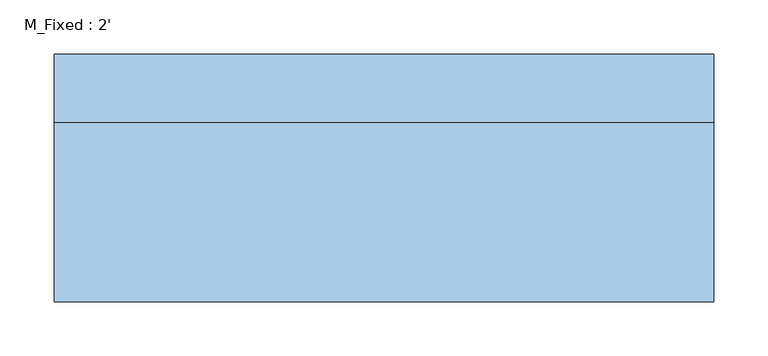
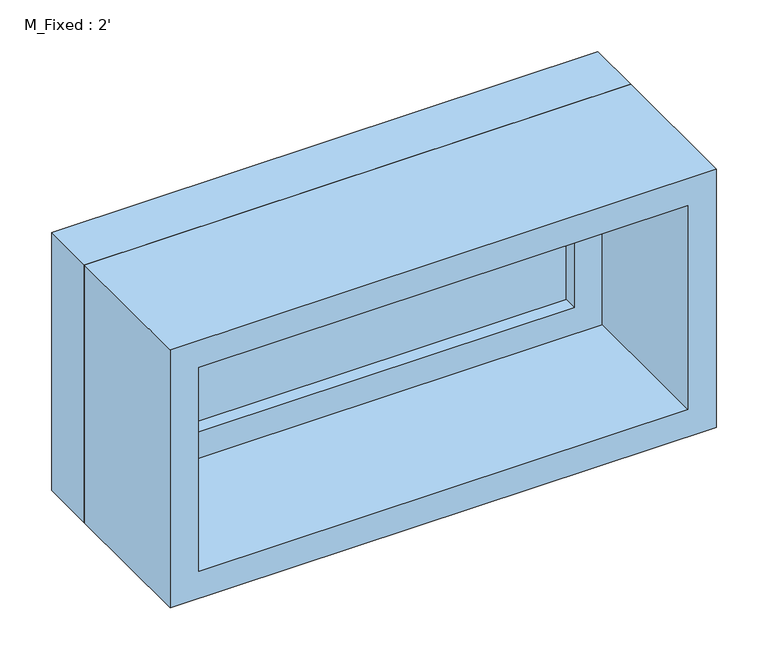
"""IFC4 building model written with IfcOpenShell, lengths in millimetres: window geometry, M_Fixed : 2'."""

from ifc_helpers import new_model, si_unit, frame, origin, place, context, project, spatial, polyline, outline, extrude, source, transform, mapped, element, save


def m_fixed_2_dd9f9b20(model_context):
    return source(origin(), model_context, "Body", "SweptSolid", [
        extrude(outline(polyline([(-241.8, 92.3), (241.8, 92.3), (241.8, 80.3), (-241.8, 80.3), (-241.8, 92.3)])), frame((0.0, 0.0, 978.0), z_axis=(0.0, 0.0, 1.0), x_axis=(1.0, 0.0, 0.0)), (0.0, 0.0, 1.0), 178.8),
        extrude(outline(polyline([(1200.8, -285.8), (934.0, -285.8), (934.0, 285.8), (1200.8, 285.8), (1200.8, -285.8)]), holes=[polyline([(1156.8, -241.8), (1156.8, 241.8), (978.0, 241.8), (978.0, -241.8), (1156.8, -241.8)])]), frame((0.0, 64.3, 0.0), z_axis=(0.0, 1.0, 0.0), x_axis=(0.0, 0.0, 1.0)), (0.0, 0.0, 1.0), 44.0),
        extrude(outline(polyline([(1219.8, -304.8), (915.0, -304.8), (915.0, 304.8), (1219.8, 304.8), (1219.8, -304.8)]), holes=[polyline([(1200.8, -285.8), (1200.8, 285.8), (934.0, 285.8), (934.0, -285.8), (1200.8, -285.8)])]), frame((0.0, 64.3, 0.0), z_axis=(0.0, 1.0, 0.0), x_axis=(0.0, 0.0, 1.0)), (0.0, 0.0, 1.0), 63.0),
        extrude(outline(polyline([(1219.8, -304.8), (915.0, -304.8), (915.0, 304.8), (1219.8, 304.8), (1219.8, -304.8)]), holes=[polyline([(1187.8, -272.8), (1187.8, 272.8), (947.0, 272.8), (947.0, -272.8), (1187.8, -272.8)])]), frame((0.0, -101.3, 0.0), z_axis=(0.0, 1.0, 0.0), x_axis=(0.0, 0.0, 1.0)), (0.0, 0.0, 1.0), 165.6),
    ])


if __name__ == "__main__":
    model = new_model("IFC4")
    model_context = context("Model", 3, world=origin())
    ifc_project = project(units=[si_unit("LENGTHUNIT", "METRE", prefix="MILLI")], contexts=[model_context])
    site = spatial("IfcSite", under=ifc_project)
    building = spatial("IfcBuilding", under=site)
    placement = place(None, origin())
    m_fixed_2_shape = m_fixed_2_dd9f9b20(model_context)
    element("IfcWindow", 1, ObjectType="M_Fixed : 2'", at=placement, inside=building, context=model_context, shape_type="MappedRepresentation", body=[
        mapped(m_fixed_2_shape, transform((0.0, 0.0, 0.0), x_axis=(1.0, 0.0, 0.0), y_axis=(0.0, 1.0, 0.0), z_axis=(0.0, 0.0, 1.0))),
    ])
    save(model, "model.ifc")

# Revit data of these elements
# Type "M_Fixed : 2'"
#   Type Mark = "32"
#   Construction Type Id = "GSP4R"
#   Analytic Construction = "1/8 in Pilkington single glazing"
#   Visual Light Transmittance = 0.9
#   Thermal Resistance (R) = 0.271106 (m²·K)/W
#   Solar Heat Gain Coefficient = 0.78
#   Heat Transfer Coefficient (U) = 3.6886 W/(m²·K)
#   Height = 1' - 0"
#   Default Sill Height = 3' - 0.02362"
#   Width = 2' - 0"
#   Window Inset = 0' - 0.74803"
#   Define Thermal Properties by = 1
#   Frame Exterior Material = Sash
#   Frame Interior Material = Sash
#   Glass Pane Material = Glass
#   Sash = Sash
#   Wall Closure = (empty or 0)
# Element 1 (IfcWindow, "M_Fixed : 2'")
#   Materials on its faces: "Sash", "Glass"
# Materials
#   "Sash": class "Wood", colour RGB 224 178 126, transparency 0, Cost = 0
#   "Glass": class "Glass", colour RGB 0 128 192, transparency 0.9, Description = "Soda Lime Glass", Cost = 0
